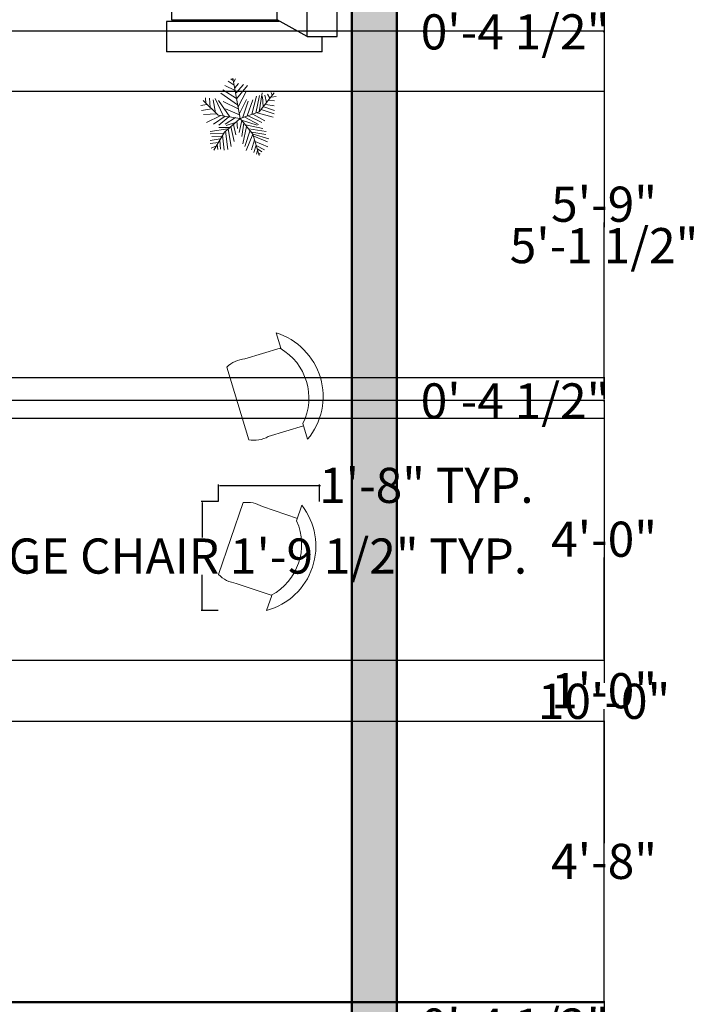
# Model space of a CAD drawing. Units: inches. Extents: x 48 to 822, y -191 to 651.
# Tile 10 of 13: x 673 to 810, y 101 to 297. Entities that reach past the tile are written whole.
import ezdxf

# ---------------------------------------------------------------- set-up
doc = ezdxf.new("R2010")
doc.units = ezdxf.units.IN
doc.header["$MEASUREMENT"] = 0
doc.layers.get('0').update_dxf_attribs({"color": 254})
for name, color, linetype, lineweight in [('A-ANNO-DIMS', 2, 'Continuous', 18), ('A-FURN', 8, 'Continuous', 18), ('A-WALL', 7, 'Continuous', 50), ('A-WALL-PATT', 8, 'Continuous', 13), ('L-PLNT', 103, 'Continuous', 18)]:
    doc.layers.add(name, color=color, linetype=linetype, lineweight=lineweight)
doc.layers.add('furniture', color=250, linetype='Continuous')
doc.styles.get("Standard").update_dxf_attribs({"font": 'arial.ttf'})
doc.dimstyles.get("Standard").update_dxf_attribs({"dimtxt": 7, "dimasz": 0.18, "dimexe": 0.18, "dimexo": 0.0625, "dimgap": 0.09, "dimtad": 0, "dimtih": 1, "dimtoh": 1, "dimzin": 0, "dimdsep": 46, "dimlunit": 3, "dimtxsty": 'Standard', "dimcen": 0.09, "dimadec": 0, "dimazin": 0, "dimtfac": 1, "dimtofl": 0, "dimtmove": 0, "dimatfit": 3, "dimfxl": 1, "dimtolj": 1, "dimtzin": 0, "dimarcsym": 0})

# ---------------------------------------------------------------- blocks, each defined once
blk = doc.blocks.new('FABRIC SOFA 4S')
at = {"layer": 'furniture'}
for p, q in [((3, 54), (34, 54)), ((3, 51), (3, 54)), ((34, 48), (34, 54)), ((0, -51), (0, 51)), ((6, 51), (0, 51)), ((6, -51), (6, 51)), ((12, 47.63), (6, 51)), ((11.14, 48), (34, 48)), ((33, 23.81), (12, 23.81)), ((33, 0), (12, 0)), ((33, -23.81), (12, -23.81)), ((6, -51), (12, -47.63)), ((11.54, -48), (34, -48)), ((34, -48), (34, -54)), ((6, -51), (0, -51)), ((3, -54), (3, -51)), ((3, -54), (34, -54))]:
    blk.add_line(p, q, dxfattribs=at)
blk.add_lwpolyline([(12, -47.63), (12, 47.63), (33, 47.63), (33, -47.63)], close=True, dxfattribs=at)
blk = doc.blocks.new('*U15')
for p, q in [((-10.186, 53.64), (-13.084, 55.962)), ((0, 0), (-10.5, 57)), ((-9.099, 51.782), (-6.563, 55.962)), ((-7.288, 39.707), (-21.778, 46.673)), ((-8.737, 47.138), (-17.069, 52.711)), ((-7.65, 43.423), (-2.578, 49.46)), ((-5.839, 35.992), (4.667, 48.067)), ((-5.114, 27.632), (10.463, 46.673)), ((-48.585, 21.131), (-49.309, 29.026)), ((-43.513, 28.561), (-42.427, 15.558)), ((-35.544, 28.097), (-24.314, 3.947)), ((-3.665, 19.273), (-27.574, 35.527)), ((-5.114, 28.097), (-24.676, 40.636)), ((-2.941, 16.486), (8.652, 37.85)), ((16.259, 5.805), (23.142, 31.348)), ((22.055, 7.198), (27.489, 32.277)), ((27, 9), (48, 36)), ((27.127, 9.056), (31.112, 35.992)), ((31.836, 30.883), (32.561, 16.486)), ((35.096, 32.741), (37.27, 22.524)), ((38.719, 34.134), (41.979, 28.561)), ((43.791, 29.954), (51.036, 30.883)), ((44.153, 36.456), (45.239, 32.741)), ((-47.498, 19.737), (-55.83, 18.344)), ((-31.5, 4.5), (-52.5, 25.5)), ((-38.442, 26.239), (-34.819, 7.663)), ((-14.533, 2.09), (-30.834, 25.31)), ((-24.314, 23.917), (-2.941, 13.7)), ((-1.129, 6.734), (9.014, 26.704)), ((3.942, 1.625), (11.187, 24.381)), ((10.101, 3.483), (17.708, 26.239)), ((33.285, 16.486), (48.862, 10.913)), ((36.183, 19.737), (48.137, 17.88)), ((40.53, 25.775), (48.862, 24.846)), ((-40.615, 13.7), (-55.105, 10.913)), ((-33.37, 6.269), (-52.207, 5.34)), ((-28.299, 3.483), (-47.86, -5.805)), ((-21.416, 3.018), (-38.079, -8.128)), ((0, 0), (-31.5, 4.5)), ((-15.982, 2.09), (-30.11, -9.521)), ((0, 0), (-22.5, -19.5)), ((-6.563, 1.161), (-21.416, -8.128)), ((-20.691, 13.7), (-1.129, 4.876)), ((0, 0), (27, 9)), ((0, 0), (18, -22.5)), ((6.478, 1.625), (26.04, -8.592)), ((11.187, 3.483), (30.749, -5.805)), ((18.07, 5.805), (35.096, -3.483)), ((24.229, 7.663), (46.688, 1.625)), ((29.662, 12.307), (48.137, 6.269)), ((-15.257, -12.772), (-30.11, -12.772)), ((-6.563, -5.805), (-19.967, -9.985)), ((-13.446, -11.378), (-8.737, -32.741)), ((-9.461, -8.592), (-6.201, -23.453)), ((-4.752, -3.483), (-3.665, -14.629)), ((2.493, -3.019), (-1.491, -20.202)), ((1.769, -2.555), (24.229, -9.521)), ((5.029, -6.27), (2.131, -25.775)), ((9.014, -11.378), (3.58, -35.992)), ((7.565, -9.056), (32.198, -14.629)), ((-17.431, -15.094), (-42.789, -18.809)), ((-24.314, -21.596), (-42.427, -22.06)), ((-26.849, -26.24), (-40.253, -25.775)), ((-22.5, -19.5), (-37.5, -45)), ((-25.038, -23.918), (-22.865, -45.281)), ((-20.691, -18.345), (-17.793, -44.352)), ((-17.069, -15.094), (-12.721, -40.172)), ((14.085, -16.951), (6.478, -40.172)), ((18.07, -22.524), (8.289, -45.745)), ((12.274, -15.094), (36.907, -18.809)), ((16.259, -19.738), (36.183, -22.989)), ((18, -22.5), (27, -52.5)), ((18.433, -22.524), (40.53, -29.026)), ((19.157, -25.311), (38.719, -33.206)), ((-28.299, -29.026), (-42.789, -31.348)), ((-30.834, -34.135), (-42.427, -35.528)), ((-34.457, -39.708), (-40.978, -42.494)), ((-32.646, -36.921), (-31.921, -44.352)), ((-29.023, -30.884), (-27.936, -43.887)), ((20.244, -30.419), (15.897, -44.816)), ((22.78, -37.85), (19.519, -48.532)), ((21.331, -32.741), (39.081, -40.636)), ((22.78, -38.314), (34.372, -44.816)), ((24.591, -45.745), (23.142, -50.854)), ((24.591, -43.423), (30.749, -47.603)), ((26.764, -49.925), (28.213, -50.854))]:
    blk.add_line(p, q)
blk = doc.blocks.new('CHAIR-LOUNGE')
for p, q in [((0, 7.16), (4.89, 21.48)), ((8.77, 20.69), (15.72, 18.31)), ((15.56, 17.83), (16.6, 20.95)), ((3.55, 5.4), (10.51, 3.03)), ((9.58, 0), (10.6, 3))]:
    blk.add_line(p, q)
for centre, radius, start, end in [((5.72, 15.59), 5.94, 59.0668, 98.0094), ((6.15, 12.8), 13.25, 284.9708, 37.976), ((5.09, 13.15), 11.48, 298.1844, 24.1095), ((4.25, 11.3), 5.94, 224.2845, 263.2272)]:
    blk.add_arc(centre, radius, start, end)
blk = doc.blocks.new('*D52')
at = {"layer": 'A-ANNO-DIMS', "color": 0, "lineweight": -2, "transparency": 16777216}
for p, q in [((713, 201.45), (709.64, 201.45)), ((709.82, 201.27), (709.82, 194.33)), ((709.82, 179.96), (709.82, 186.9)), ((713, 179.78), (709.64, 179.78))]:
    blk.add_line(p, q, dxfattribs=at)
at = {"layer": 'A-ANNO-DIMS', "color": 0, "transparency": 16777216}
for points in [[(709.79, 201.27), (709.85, 201.27), (709.82, 201.45)], [(709.79, 179.96), (709.85, 179.96), (709.82, 179.78)]]:
    blk.add_solid(points, dxfattribs=at)
at = {"layer": 'Defpoints', "color": 0, "transparency": 16777216}
for p in [(709.82, 201.45), (713.07, 201.45), (713.07, 179.78)]:
    blk.add_point(p, dxfattribs=at)
at = {"layer": 'A-ANNO-DIMS', "color": 0, "transparency": 16777216, "insert": (709.82, 190.62), "char_height": 7, "attachment_point": 5}
blk.add_mtext('\\A1;LOUNGE CHAIR 1\'-9 1/2" TYP.', dxfattribs=at)
blk = doc.blocks.new('*D53')
at = {"layer": 'A-ANNO-DIMS', "color": 0, "lineweight": -2, "transparency": 16777216}
for p, q in [((713.07, 201.51), (713.07, 204.88)), ((713.25, 204.7), (733.01, 204.7)), ((733.19, 201.51), (733.19, 204.88)), ((733.19, 204.7), (733.37, 204.7))]:
    blk.add_line(p, q, dxfattribs=at)
at = {"layer": 'A-ANNO-DIMS', "color": 0, "transparency": 16777216}
for points in [[(713.25, 204.73), (713.25, 204.67), (713.07, 204.7)], [(733.01, 204.73), (733.01, 204.67), (733.19, 204.7)]]:
    blk.add_solid(points, dxfattribs=at)
at = {"layer": 'Defpoints', "color": 0, "transparency": 16777216}
for p in [(733.19, 204.7), (713.07, 201.45), (733.19, 201.45)]:
    blk.add_point(p, dxfattribs=at)
at = {"layer": 'A-ANNO-DIMS', "color": 0, "transparency": 16777216, "insert": (754.47, 204.7), "char_height": 7, "attachment_point": 5}
blk.add_mtext('\\A1;1\'-8" TYP.', dxfattribs=at)
blk = doc.blocks.new('*D85')
at = {"layer": 'A-ANNO-DIMS', "color": 0, "lineweight": -2, "transparency": 16777216}
for p, q in [((321.36, 283.18), (790.04, 283.18)), ((789.86, 283), (789.86, 256.14)), ((789.86, 221.87), (789.86, 248.73)), ((321.2, 221.69), (790.04, 221.69))]:
    blk.add_line(p, q, dxfattribs=at)
at = {"layer": 'A-ANNO-DIMS', "color": 0, "transparency": 16777216}
for points in [[(789.83, 283), (789.89, 283), (789.86, 283.18)], [(789.83, 221.87), (789.89, 221.87), (789.86, 221.69)]]:
    blk.add_solid(points, dxfattribs=at)
at = {"layer": 'Defpoints', "color": 0, "transparency": 16777216}
for p in [(321.3, 283.18), (321.14, 221.69), (789.86, 221.69)]:
    blk.add_point(p, dxfattribs=at)
at = {"layer": 'A-ANNO-DIMS', "color": 0, "transparency": 16777216, "insert": (789.86, 252.44), "char_height": 7, "attachment_point": 5}
blk.add_mtext('\\A1;5\'-1 1/2"', dxfattribs=at)
blk = doc.blocks.new('*D110')
at = {"layer": 'A-ANNO-DIMS', "color": 0, "lineweight": -2, "transparency": 16777216}
for p, q in [((517.67, 299.69), (790.04, 299.69)), ((789.86, 299.51), (789.86, 295.37)), ((517.67, 295.19), (790.04, 295.19)), ((789.86, 295.01), (789.68, 295.01)), ((789.86, 295.19), (789.86, 295.01))]:
    blk.add_line(p, q, dxfattribs=at)
at = {"layer": 'A-ANNO-DIMS', "color": 0, "transparency": 16777216}
for points in [[(789.83, 299.51), (789.89, 299.51), (789.86, 299.69)], [(789.83, 295.37), (789.89, 295.37), (789.86, 295.19)]]:
    blk.add_solid(points, dxfattribs=at)
at = {"layer": 'Defpoints', "color": 0, "transparency": 16777216}
for p in [(517.61, 299.69), (517.61, 295.19), (789.86, 295.19)]:
    blk.add_point(p, dxfattribs=at)
at = {"layer": 'A-ANNO-DIMS', "color": 0, "transparency": 16777216, "insert": (772.13, 295.01), "char_height": 7, "attachment_point": 5}
blk.add_mtext('\\A1;0\'-4 1/2"', dxfattribs=at)
blk = doc.blocks.new('*D111')
at = {"layer": 'A-ANNO-DIMS', "color": 0, "lineweight": -2, "transparency": 16777216}
for p, q in [((517.67, 295.19), (790.04, 295.19)), ((789.86, 295.01), (789.86, 264.35)), ((789.86, 226.37), (789.86, 257.02)), ((517.67, 226.19), (790.04, 226.19))]:
    blk.add_line(p, q, dxfattribs=at)
at = {"layer": 'A-ANNO-DIMS', "color": 0, "transparency": 16777216}
for points in [[(789.83, 295.01), (789.89, 295.01), (789.86, 295.19)], [(789.83, 226.37), (789.89, 226.37), (789.86, 226.19)]]:
    blk.add_solid(points, dxfattribs=at)
at = {"layer": 'Defpoints', "color": 0, "transparency": 16777216}
for p in [(517.61, 295.19), (517.61, 226.19), (789.86, 226.19)]:
    blk.add_point(p, dxfattribs=at)
at = {"layer": 'A-ANNO-DIMS', "color": 0, "transparency": 16777216, "insert": (789.86, 260.69), "char_height": 7, "attachment_point": 5}
blk.add_mtext('\\A1;5\'-9"', dxfattribs=at)
blk = doc.blocks.new('*D112')
at = {"layer": 'A-ANNO-DIMS', "color": 0, "lineweight": -2, "transparency": 16777216}
for p, q in [((517.67, 226.19), (790.04, 226.19)), ((789.86, 226.01), (789.86, 221.87)), ((517.67, 221.69), (790.04, 221.69)), ((789.86, 221.69), (789.86, 221.51)), ((789.86, 221.51), (789.68, 221.51))]:
    blk.add_line(p, q, dxfattribs=at)
at = {"layer": 'A-ANNO-DIMS', "color": 0, "transparency": 16777216}
for points in [[(789.83, 226.01), (789.89, 226.01), (789.86, 226.19)], [(789.83, 221.87), (789.89, 221.87), (789.86, 221.69)]]:
    blk.add_solid(points, dxfattribs=at)
at = {"layer": 'Defpoints', "color": 0, "transparency": 16777216}
for p in [(517.61, 226.19), (517.61, 221.69), (789.86, 221.69)]:
    blk.add_point(p, dxfattribs=at)
at = {"layer": 'A-ANNO-DIMS', "color": 0, "transparency": 16777216, "insert": (772.13, 221.51), "char_height": 7, "attachment_point": 5}
blk.add_mtext('\\A1;0\'-4 1/2"', dxfattribs=at)
blk = doc.blocks.new('*D113')
at = {"layer": 'A-ANNO-DIMS', "color": 0, "lineweight": -2, "transparency": 16777216}
for p, q in [((517.67, 221.69), (790.04, 221.69)), ((789.86, 221.51), (789.86, 165.35)), ((789.86, 101.87), (789.86, 158.02)), ((517.67, 101.69), (790.04, 101.69))]:
    blk.add_line(p, q, dxfattribs=at)
at = {"layer": 'A-ANNO-DIMS', "color": 0, "transparency": 16777216}
for points in [[(789.83, 221.51), (789.89, 221.51), (789.86, 221.69)], [(789.83, 101.87), (789.89, 101.87), (789.86, 101.69)]]:
    blk.add_solid(points, dxfattribs=at)
at = {"layer": 'Defpoints', "color": 0, "transparency": 16777216}
for p in [(517.61, 221.69), (517.61, 101.69), (789.86, 101.69)]:
    blk.add_point(p, dxfattribs=at)
at = {"layer": 'A-ANNO-DIMS', "color": 0, "transparency": 16777216, "insert": (789.86, 161.69), "char_height": 7, "attachment_point": 5}
blk.add_mtext('\\A1;10\'-0"', dxfattribs=at)
blk = doc.blocks.new('*D114')
at = {"layer": 'A-ANNO-DIMS', "color": 0, "lineweight": -2, "transparency": 16777216}
for p, q in [((517.67, 101.69), (790.04, 101.69)), ((789.86, 101.51), (789.86, 97.37)), ((517.67, 97.19), (790.04, 97.19)), ((789.86, 97.01), (789.68, 97.01)), ((789.86, 97.19), (789.86, 97.01))]:
    blk.add_line(p, q, dxfattribs=at)
at = {"layer": 'A-ANNO-DIMS', "color": 0, "transparency": 16777216}
for points in [[(789.83, 101.51), (789.89, 101.51), (789.86, 101.69)], [(789.83, 97.37), (789.89, 97.37), (789.86, 97.19)]]:
    blk.add_solid(points, dxfattribs=at)
at = {"layer": 'Defpoints', "color": 0, "transparency": 16777216}
for p in [(517.61, 101.69), (517.61, 97.19), (789.86, 97.19)]:
    blk.add_point(p, dxfattribs=at)
at = {"layer": 'A-ANNO-DIMS', "color": 0, "transparency": 16777216, "insert": (772.13, 97.01), "char_height": 7, "attachment_point": 5}
blk.add_mtext('\\A1;0\'-4 1/2"', dxfattribs=at)
blk = doc.blocks.new('*D127')
at = {"layer": 'A-ANNO-DIMS', "color": 0, "lineweight": -2, "transparency": 16777216}
for p, q in [((659.17, 218.07), (790.04, 218.07)), ((789.86, 217.89), (789.86, 197.63)), ((789.86, 170.05), (789.86, 190.31)), ((659.17, 169.87), (790.04, 169.87))]:
    blk.add_line(p, q, dxfattribs=at)
at = {"layer": 'A-ANNO-DIMS', "color": 0, "transparency": 16777216}
for points in [[(789.83, 217.89), (789.89, 217.89), (789.86, 218.07)], [(789.83, 170.05), (789.89, 170.05), (789.86, 169.87)]]:
    blk.add_solid(points, dxfattribs=at)
at = {"layer": 'Defpoints', "color": 0, "transparency": 16777216}
for p in [(659.11, 218.07), (659.11, 169.87), (789.86, 169.87)]:
    blk.add_point(p, dxfattribs=at)
at = {"layer": 'A-ANNO-DIMS', "color": 0, "transparency": 16777216, "insert": (789.86, 193.97), "char_height": 7, "attachment_point": 5}
blk.add_mtext('\\A1;4\'-0"', dxfattribs=at)
blk = doc.blocks.new('*D128')
at = {"layer": 'A-ANNO-DIMS', "color": 0, "lineweight": -2, "transparency": 16777216}
for p, q in [((659.17, 169.87), (790.04, 169.87)), ((789.86, 169.69), (789.86, 167.46)), ((789.86, 157.9), (789.86, 160.13)), ((659.17, 157.72), (790.04, 157.72))]:
    blk.add_line(p, q, dxfattribs=at)
at = {"layer": 'A-ANNO-DIMS', "color": 0, "transparency": 16777216}
for points in [[(789.83, 169.69), (789.89, 169.69), (789.86, 169.87)], [(789.83, 157.9), (789.89, 157.9), (789.86, 157.72)]]:
    blk.add_solid(points, dxfattribs=at)
at = {"layer": 'Defpoints', "color": 0, "transparency": 16777216}
for p in [(659.11, 169.87), (659.11, 157.72), (789.86, 157.72)]:
    blk.add_point(p, dxfattribs=at)
at = {"layer": 'A-ANNO-DIMS', "color": 0, "transparency": 16777216, "insert": (789.86, 163.8), "char_height": 7, "attachment_point": 5}
blk.add_mtext('\\A1;1\'-0"', dxfattribs=at)
blk = doc.blocks.new('*D129')
at = {"layer": 'A-ANNO-DIMS', "color": 0, "lineweight": -2, "transparency": 16777216}
for p, q in [((659.17, 157.72), (790.04, 157.72)), ((789.86, 157.54), (789.86, 133.47)), ((789.86, 102.08), (789.86, 126.14)), ((659.17, 101.9), (790.04, 101.9))]:
    blk.add_line(p, q, dxfattribs=at)
at = {"layer": 'A-ANNO-DIMS', "color": 0, "transparency": 16777216}
for points in [[(789.83, 157.54), (789.89, 157.54), (789.86, 157.72)], [(789.83, 102.08), (789.89, 102.08), (789.86, 101.9)]]:
    blk.add_solid(points, dxfattribs=at)
at = {"layer": 'Defpoints', "color": 0, "transparency": 16777216}
for p in [(659.11, 157.72), (659.11, 101.9), (789.86, 101.9)]:
    blk.add_point(p, dxfattribs=at)
at = {"layer": 'A-ANNO-DIMS', "color": 0, "transparency": 16777216, "insert": (789.86, 129.81), "char_height": 7, "attachment_point": 5}
blk.add_mtext('\\A1;4\'-8"', dxfattribs=at)
blk = doc.blocks.new('*D130')
at = {"layer": 'A-ANNO-DIMS', "color": 0, "lineweight": -2, "transparency": 16777216}
for p, q in [((659.17, 101.9), (790.04, 101.9)), ((789.86, 101.72), (789.86, 69.94)), ((789.86, 30.74), (789.86, 62.52)), ((659.17, 30.56), (790.04, 30.56))]:
    blk.add_line(p, q, dxfattribs=at)
at = {"layer": 'A-ANNO-DIMS', "color": 0, "transparency": 16777216}
for points in [[(789.83, 101.72), (789.89, 101.72), (789.86, 101.9)], [(789.83, 30.74), (789.89, 30.74), (789.86, 30.56)]]:
    blk.add_solid(points, dxfattribs=at)
at = {"layer": 'Defpoints', "color": 0, "transparency": 16777216}
for p in [(659.11, 101.9), (659.11, 30.56), (789.86, 30.56)]:
    blk.add_point(p, dxfattribs=at)
at = {"layer": 'A-ANNO-DIMS', "color": 0, "transparency": 16777216, "insert": (789.86, 66.23), "char_height": 7, "attachment_point": 5}
blk.add_mtext('\\A1;5\'-11 1/2"', dxfattribs=at)

msp = doc.modelspace()

# ---------------------------------------------------------------- hatches: boundary and pattern name
at = {"layer": 'A-WALL-PATT'}
h = msp.add_hatch(color=256, dxfattribs=at)
h.dxf.hatch_style = 1
h.paths.add_polyline_path([(614.11, 432.437), (609.61, 432.437), (609.61, 376.187), (535.284, 376.187), (535.284, 371.687), (547.61, 371.687), (547.61, 359.12), (552.11, 359.12), (552.11, 371.687), (609.61, 371.687), (609.61, 335.687), (614.11, 335.687)], flags=17)
h.paths.add_polyline_path([(614.11, 434.687), (609.61, 434.687), (609.61, 432.437), (614.11, 432.437)], flags=17)
h.paths.add_polyline_path([(573.934, 434.687), (517.61, 434.687), (517.61, 590.687), (650.61, 590.687), (650.61, 585.522), (655.11, 585.522), (655.11, 590.687), (739.61, 590.687), (739.61, 548.687), (655.11, 548.687), (655.11, 550.72), (650.61, 550.72), (650.61, 458.608), (655.11, 458.608), (655.11, 544.187), (739.61, 544.187), (739.61, 434.541), (650.61, 434.541), (650.61, 430.041), (739.61, 430.041), (739.61, -16.844), (729.973, -16.844), (729.973, -21.344), (748.61, -21.344), (748.61, 599.687), (508.61, 599.687), (508.61, -120.313), (543.114, -120.313), (543.114, -111.313), (517.61, -111.313), (517.61, 38.687), (607.29, 38.687), (607.29, 43.187), (517.61, 43.187), (517.61, 97.187), (654.61, 97.187), (654.61, 30.562), (659.11, 30.562), (659.11, 101.895), (654.61, 101.895), (654.61, 101.687), (517.61, 101.687), (517.61, 221.687), (654.61, 221.687), (654.61, 218.066), (659.11, 218.066), (659.11, 226.187), (517.61, 226.187), (517.61, 295.187), (614.11, 295.187), (648.087, 295.187), (661.07, 295.187), (661.07, 299.687), (614.11, 299.687), (552.11, 299.687), (552.11, 341.37), (547.61, 341.37), (547.61, 299.687), (517.61, 299.687), (517.61, 371.687), (517.534, 371.687), (517.534, 376.187), (517.61, 430.187), (573.934, 430.187)])
h.paths.add_polyline_path([(659.11, -87.328), (654.61, -87.328), (654.61, -111.313), (598.94, -111.313), (598.94, -120.313), (659.11, -120.313)], flags=0)
h.paths.add_polyline_path([(671.266, -16.844), (659.11, -16.844), (659.11, -12.05), (654.61, -12.05), (654.61, -31.502), (659.11, -31.502), (659.11, -21.344), (671.266, -21.344)], flags=17)
h.paths.add_polyline_path([(606.11, 97.187), (601.61, 97.187), (601.61, 75.902), (606.11, 75.902)], flags=17)
h.paths.add_polyline_path([(659.11, 169.875), (654.61, 169.875), (654.61, 157.721), (659.11, 157.721)], flags=17)

# ---------------------------------------------------------------- linework, layer by layer
at = {"layer": 'A-WALL'}
for p, q in [((748.61, 599.687), (748.61, -120.313)), ((739.61, 430.041), (739.61, -16.844))]:
    msp.add_line(p, q, dxfattribs=at)

# ---------------------------------------------------------------- block references
at = {"layer": 'A-FURN', "xscale": -1}
msp.add_blockref('FABRIC SOFA 4S', (736.72, 345.068), dxfattribs=at)
at = {"layer": 'A-FURN', "extrusion": (0, 0, -1), "zscale": -1, "rotation": 182.0533150846993}
msp.add_blockref('CHAIR-LOUNGE', (-714.966, 235.4), dxfattribs=at)
at = {"layer": 'A-FURN'}
msp.add_blockref('CHAIR-LOUNGE', (713.065, 179.783), dxfattribs=at)
at = {"layer": 'L-PLNT', "xscale": 0.1404061648656346, "yscale": 0.1404061648656346, "zscale": 0.1404061648656346}
msp.add_blockref('*U15', (717.391, 277.791), dxfattribs=at)

# ---------------------------------------------------------------- dimensions: what is measured, and where the dimension line sits
at = {"layer": 'A-ANNO-DIMS'}
for base, p1, p2, picture, middle in [((789.86, 295.187), (517.61, 299.687), (517.61, 295.187), '*D110', (772.131, 295.007)), ((789.86, 226.187), (517.61, 295.187), (517.61, 226.187), '*D111', (789.86, 260.687)), ((789.86, 221.687), (321.299, 283.184), (321.136, 221.687), '*D85', (789.86, 252.435)), ((789.86, 221.687), (517.61, 226.187), (517.61, 221.687), '*D112', (772.131, 221.507)), ((789.86, 101.687), (517.61, 221.687), (517.61, 101.687), '*D113', (789.86, 161.687)), ((789.86, 169.875), (659.11, 218.066), (659.11, 169.875), '*D127', (789.86, 193.97)), ((789.86, 157.721), (659.11, 169.875), (659.11, 157.721), '*D128', (789.86, 163.798)), ((789.86, 101.895), (659.11, 157.721), (659.11, 101.895), '*D129', (789.86, 129.808)), ((789.86, 97.187), (517.61, 101.687), (517.61, 97.187), '*D114', (772.131, 97.007)), ((789.86, 30.562), (659.11, 101.895), (659.11, 30.562), '*D130', (789.86, 66.229))]:
    dim = msp.add_linear_dim(base=base, p1=p1, p2=p2, angle=90, dimstyle='Standard', override={"dimdec": 1, "dimlfac": 1, "dimrnd": 0, "dimzin": 1, "dimdsep": 46, "dimlunit": 4, "dimfrac": 2}, dxfattribs=at)
    dim.commit()
    dim.dimension.update_dxf_attribs({"geometry": picture, "text_midpoint": middle})
dim = msp.add_linear_dim(base=(709.815, 201.449), p1=(713.065, 179.783), p2=(713.065, 201.449), angle=90, text='LOUNGE CHAIR <> TYP.', dimstyle='Standard', override={"dimdec": 1, "dimlfac": 1, "dimrnd": 0, "dimzin": 1, "dimdsep": 46, "dimlunit": 4, "dimfrac": 2}, dxfattribs=at)
dim.commit()
dim.dimension.update_dxf_attribs({"geometry": '*D52', "text_midpoint": (709.815, 190.616)})
dim = msp.add_linear_dim(base=(733.192, 204.698), p1=(713.065, 201.449), p2=(733.192, 201.449), text='<> TYP.', dimstyle='Standard', override={"dimdec": 1, "dimlfac": 1, "dimrnd": 0, "dimzin": 1, "dimdsep": 46, "dimlunit": 4, "dimfrac": 2}, dxfattribs=at)
dim.commit()
dim.dimension.update_dxf_attribs({"geometry": '*D53', "text_midpoint": (754.467, 204.698)})

doc.saveas('drawing.dxf')
